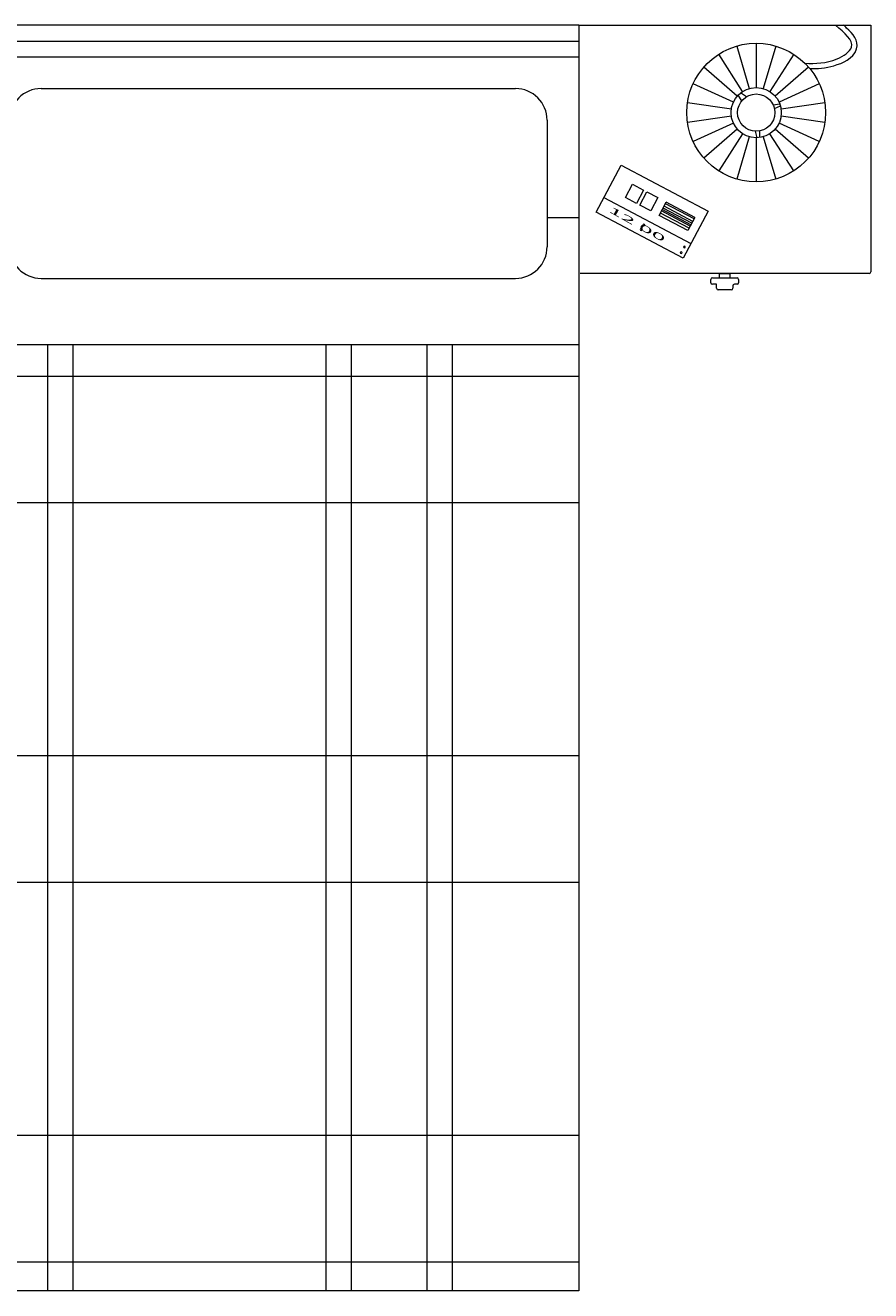
# Model space of a CAD drawing. Units: inches. Extents: x 1994 to 3075, y 3517 to 3950.
# Tile 24 of 58: x 1994.29701 to 1994.34963, y 3553.80439 to 3553.88313. Entities that reach past the tile are written whole.
import ezdxf

# ---------------------------------------------------------------- set-up
doc = ezdxf.new("R2010")
doc.units = ezdxf.units.IN
doc.layers.add('A-FURN-REFR', color=8, linetype='Continuous', lineweight=13)
doc.layers.add('A-FURN-REFR-TEXT', color=7, linetype='Continuous', lineweight=13)
doc.styles.get("Standard").update_dxf_attribs({"font": 'arial.ttf'})

msp = doc.modelspace()

# ---------------------------------------------------------------- linework, layer by layer
at = {"layer": 'A-FURN-REFR'}
for p, q in [((1994.331458, 3553.883133), (1994.260591, 3553.883133)), ((1994.331458, 3553.883133), (1994.331458, 3553.804393)), ((1994.331458, 3553.883133), (1994.349631, 3553.883133)), ((1994.331458, 3553.883133), (1994.349631, 3553.883133)), ((1994.349631, 3553.883133), (1994.349631, 3553.867783)), ((1994.260591, 3553.882149), (1994.331458, 3553.882149)), ((1994.342504, 3553.882018), (1994.342504, 3553.879265)), ((1994.342504, 3553.882018), (1994.342504, 3553.879265)), ((1994.260591, 3553.881165), (1994.331458, 3553.881165)), ((1994.341658, 3553.879016), (1994.34017, 3553.881332)), ((1994.341288, 3553.881843), (1994.342063, 3553.879201)), ((1994.34372, 3553.881843), (1994.342944, 3553.879201)), ((1994.344837, 3553.881332), (1994.343349, 3553.879016)), ((1994.341322, 3553.878725), (1994.339242, 3553.880528)), ((1994.345766, 3553.880528), (1994.343685, 3553.878725)), ((1994.297993, 3553.879196), (1994.327521, 3553.879196)), ((1994.341081, 3553.878351), (1994.338577, 3553.879494)), ((1994.341609, 3553.878437), (1994.341385, 3553.878793)), ((1994.341892, 3553.878685), (1994.341534, 3553.878928)), ((1994.34643, 3553.879494), (1994.343926, 3553.878351)), ((1994.340956, 3553.877924), (1994.338231, 3553.878315)), ((1994.343556, 3553.878186), (1994.343966, 3553.878254)), ((1994.343635, 3553.87795), (1994.344011, 3553.878116)), ((1994.346776, 3553.878315), (1994.344051, 3553.877924)), ((1994.329489, 3553.877228), (1994.329489, 3553.869354)), ((1994.340956, 3553.877479), (1994.338231, 3553.877087)), ((1994.346776, 3553.877087), (1994.344051, 3553.877479)), ((1994.341081, 3553.877052), (1994.338577, 3553.875908)), ((1994.341322, 3553.876677), (1994.339242, 3553.874874)), ((1994.341658, 3553.876386), (1994.34017, 3553.87407)), ((1994.342446, 3553.876544), (1994.342548, 3553.876138)), ((1994.342714, 3553.876562), (1994.342711, 3553.876152)), ((1994.344837, 3553.87407), (1994.343349, 3553.876386)), ((1994.345766, 3553.874874), (1994.343685, 3553.876677)), ((1994.34643, 3553.875908), (1994.343926, 3553.877052)), ((1994.342063, 3553.876201), (1994.341288, 3553.87356)), ((1994.342504, 3553.876138), (1994.342504, 3553.873385)), ((1994.342504, 3553.876138), (1994.342504, 3553.873385)), ((1994.342944, 3553.876201), (1994.34372, 3553.87356)), ((1994.332541, 3553.871507), (1994.334095, 3553.874439)), ((1994.334095, 3553.874439), (1994.339504, 3553.871572)), ((1994.334371, 3553.872414), (1994.334809, 3553.87324)), ((1994.334809, 3553.87324), (1994.335493, 3553.872877)), ((1994.335493, 3553.872877), (1994.335055, 3553.872052)), ((1994.335252, 3553.871948), (1994.33569, 3553.872773)), ((1994.33569, 3553.872773), (1994.336373, 3553.872411)), ((1994.333025, 3553.872421), (1994.338434, 3553.869553)), ((1994.335055, 3553.872052), (1994.334371, 3553.872414)), ((1994.335936, 3553.871585), (1994.335252, 3553.871948)), ((1994.336373, 3553.872411), (1994.335936, 3553.871585)), ((1994.336467, 3553.871303), (1994.336905, 3553.872129)), ((1994.338444, 3553.870718), (1994.336659, 3553.871664)), ((1994.338496, 3553.870816), (1994.336711, 3553.871763)), ((1994.338556, 3553.870928), (1994.33677, 3553.871874)), ((1994.338639, 3553.871084), (1994.336853, 3553.872031)), ((1994.338691, 3553.871182), (1994.336905, 3553.872129)), ((1994.329489, 3553.871179), (1994.331458, 3553.871179)), ((1994.33795, 3553.868639), (1994.332541, 3553.871507)), ((1994.338253, 3553.870357), (1994.336467, 3553.871303)), ((1994.338329, 3553.870501), (1994.336543, 3553.871447)), ((1994.3384, 3553.870633), (1994.336614, 3553.87158)), ((1994.339504, 3553.871572), (1994.33795, 3553.868639)), ((1994.338691, 3553.871182), (1994.338253, 3553.870357)), ((1994.297993, 3553.867385), (1994.327521, 3553.867385)), ((1994.349536, 3553.867689), (1994.331552, 3553.867689)), ((1994.339682, 3553.867113), (1994.339682, 3553.867324)), ((1994.339777, 3553.867418), (1994.341311, 3553.867418)), ((1994.340039, 3553.867019), (1994.339777, 3553.867019)), ((1994.340039, 3553.866767), (1994.340039, 3553.867019)), ((1994.340225, 3553.867418), (1994.340225, 3553.867689)), ((1994.340225, 3553.867689), (1994.340863, 3553.867689)), ((1994.340863, 3553.867689), (1994.340863, 3553.867418)), ((1994.341311, 3553.867019), (1994.341144, 3553.867019)), ((1994.341406, 3553.867324), (1994.341406, 3553.867113)), ((1994.340955, 3553.866672), (1994.340133, 3553.866672)), ((1994.341049, 3553.866924), (1994.341049, 3553.866767)), ((1994.260591, 3553.863279), (1994.331458, 3553.863279)), ((1994.298387, 3553.863279), (1994.298387, 3553.804393)), ((1994.299961, 3553.863279), (1994.299961, 3553.804393)), ((1994.315709, 3553.863279), (1994.315709, 3553.804393)), ((1994.317284, 3553.863279), (1994.317284, 3553.804393)), ((1994.322009, 3553.863279), (1994.322009, 3553.804393)), ((1994.323584, 3553.863279), (1994.323584, 3553.804393)), ((1994.260591, 3553.861311), (1994.331458, 3553.861311)), ((1994.260591, 3553.853437), (1994.331458, 3553.853437)), ((1994.260591, 3553.837689), (1994.331458, 3553.837689)), ((1994.260591, 3553.829815), (1994.331458, 3553.829815)), ((1994.260591, 3553.814067), (1994.331458, 3553.814067)), ((1994.260591, 3553.806193), (1994.331458, 3553.806193)), ((1994.331458, 3553.804393), (1994.260591, 3553.804393))]:
    msp.add_line(p, q, dxfattribs=at)
for radius in [0.004316, 0.001563, 0.001158]:
    msp.add_circle((1994.342504, 3553.877701), radius, dxfattribs=at)
for centre, radius, start, end in [((1994.297993, 3553.877228), 0.001969, 90, 180), ((1994.327521, 3553.877228), 0.001969, 0, 90), ((1994.335339, 3553.870425), 0.0000554, 90, 270), ((1994.335339, 3553.870425), 0.0000554, 270, 90), ((1994.335511, 3553.870705), 0.0000554, 90, 270), ((1994.335511, 3553.870705), 0.0000554, 270, 90), ((1994.297993, 3553.869354), 0.001969, 180, 270), ((1994.327521, 3553.869354), 0.001969, 270, 0), ((1994.338036, 3553.869337), 0.0000554, 90, 270), ((1994.338036, 3553.869337), 0.0000554, 270, 90), ((1994.337836, 3553.868987), 0.0000554, 90, 270), ((1994.337836, 3553.868987), 0.0000554, 270, 90), ((1994.349536, 3553.867783), 0.0000945, 270, 0), ((1994.339777, 3553.867324), 0.0000945, 90, 180), ((1994.339777, 3553.867113), 0.0000945, 180, 270), ((1994.341144, 3553.866924), 0.0000945, 90, 180), ((1994.341311, 3553.867324), 0.0000945, 0, 90), ((1994.341311, 3553.867113), 0.0000945, 270, 0), ((1994.340133, 3553.866767), 0.0000945, 180, 270), ((1994.340955, 3553.866767), 0.0000945, 270, 0)]:
    msp.add_arc(centre, radius, start, end, dxfattribs=at)
for points, knots in [([(1994.345541, 3553.880768), (1994.346194, 3553.880756), (1994.347216, 3553.880749), (1994.348944, 3553.881874), (1994.348, 3553.882666), (1994.347434, 3553.883133)], [0, 0, 0, 0, 0.002019468, 0.003165929, 0.004854689, 0.004854689, 0.004854689, 0.004854689]), ([(1994.345841, 3553.880438), (1994.346314, 3553.880434), (1994.346815, 3553.880455), (1994.347881, 3553.880788), (1994.348554, 3553.88104), (1994.348915, 3553.882194), (1994.348515, 3553.882614), (1994.34807, 3553.883022), (1994.348006, 3553.883078), (1994.347942, 3553.883133)], [0.0077183, 0.0077183, 0.0077183, 0.0077183, 0.0428867, 0.0428867, 0.0785443, 0.0785443, 0.1084778, 0.1084778, 0.1132873, 0.1132873, 0.1132873, 0.1132873])]:
    msp.add_open_spline(points, degree=3, knots=knots, dxfattribs=at)

# ---------------------------------------------------------------- texts
at = {"layer": 'A-FURN-REFR-TEXT', "width": 3}
msp.add_text('12 00', height=0.0003958, rotation=330.64352, dxfattribs=at).set_placement((1994.333268, 3553.87156))

doc.saveas('drawing.dxf')
